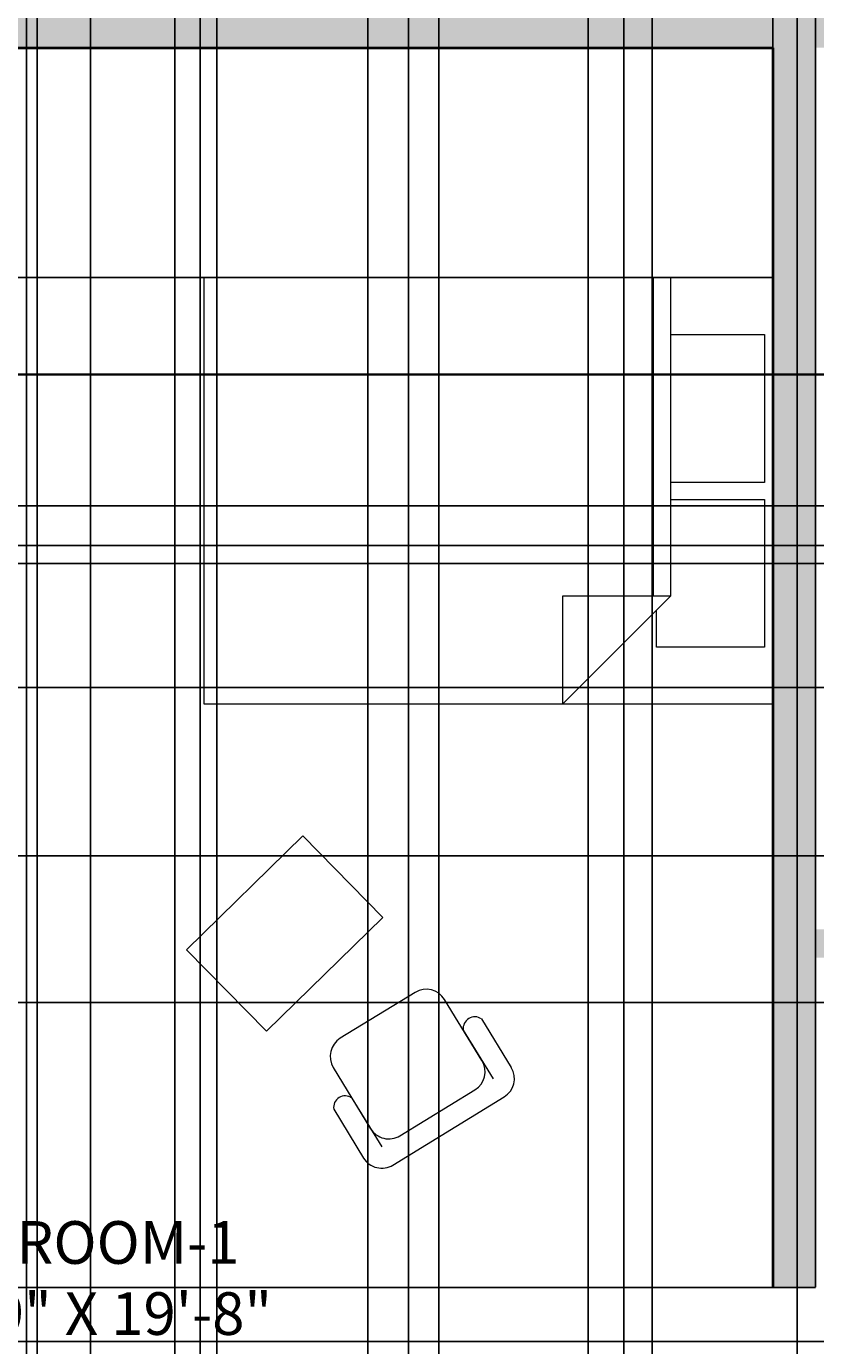
# Model space of a CAD drawing. Units: inches. Extents: x 818 to 1898, y 976 to 2364.
# Tile 43 of 96: x 1512 to 1623, y 1409 to 1594. Entities that reach past the tile are written whole.
import ezdxf

# ---------------------------------------------------------------- set-up
doc = ezdxf.new("R2010")
doc.units = ezdxf.units.IN
doc.header["$LTSCALE"] = 5
doc.header["$MEASUREMENT"] = 0
for name, color, linetype, lineweight in [('A-ANNO-DIMS', 2, 'Continuous', 18), ('A-AREA-IDEN', 7, 'Continuous', 18), ('A-DOOR', 3, 'Continuous', 25), ('A-FURN', 8, 'Continuous', 18), ('A-WALL', 7, 'Continuous', 40)]:
    doc.layers.add(name, color=color, linetype=linetype, lineweight=lineweight)
doc.layers.add('A-WALL-PATT', color=251, linetype='Continuous', lineweight=13, true_color=0x636466)
doc.styles.get("Standard").update_dxf_attribs({"font": 'arial.ttf'})
doc.dimstyles.get("Standard").update_dxf_attribs({"dimtxt": 0.18, "dimasz": 0.18, "dimexe": 0.18, "dimexo": 0.0625, "dimgap": 0.09, "dimtad": 0, "dimtih": 1, "dimtoh": 1, "dimdec": 4, "dimzin": 0, "dimdsep": 46, "dimtxsty": 'Standard', "dimcen": 0.09, "dimadec": 0, "dimazin": 0, "dimtfac": 1, "dimtdec": 4, "dimtofl": 0, "dimtmove": 0, "dimatfit": 3, "dimfxl": 1, "dimtolj": 1, "dimtzin": 0, "dimarcsym": 0})

# ---------------------------------------------------------------- blocks, each defined once
blk = doc.blocks.new('Bed - Queen')
for p, q in [((0, -80.00003), (0, 0)), ((0, 0), (59.99999, 0)), ((59.99999, 0), (59.99999, -80.00003)), ((7.99999, -1.2), (28.79998, -1.2)), ((7.99999, -14.4), (7.99999, -1.2)), ((28.79998, -1.2), (28.79998, -14.4)), ((31.19999, -1.2), (51.99999, -1.2)), ((31.19999, -14.4), (31.19999, -1.2)), ((51.99999, -1.2), (51.99999, -16.4)), ((0, -14.4), (44.8, -14.4)), ((59.99999, -29.6), (44.8, -14.4)), ((44.8, -14.4), (44.8, -29.6)), ((51.99999, -16.4), (46.79936, -16.4)), ((44.8, -16.8), (0, -16.8)), ((44.8, -29.6), (59.99999, -29.6)), ((59.99999, -80.00003), (0, -80.00003))]:
    blk.add_line(p, q)
blk = doc.blocks.new('*D101')
at = {"layer": 'A-ANNO-DIMS', "color": 0, "lineweight": -2, "ltscale": 5, "transparency": 16777216}
for p, q in [((1507.3, 1071.12), (1507.3, 2363.87)), ((1507.48, 2363.69), (1536, 2363.69)), ((1565.3, 2363.69), (1536.78, 2363.69)), ((1565.48, 1071.12), (1565.48, 2363.87))]:
    blk.add_line(p, q, dxfattribs=at)
at = {"layer": 'A-ANNO-DIMS', "color": 0, "ltscale": 5, "transparency": 16777216}
for points in [[(1507.48, 2363.72), (1507.48, 2363.66), (1507.3, 2363.69)], [(1565.3, 2363.72), (1565.3, 2363.66), (1565.48, 2363.69)]]:
    blk.add_solid(points, dxfattribs=at)
at = {"layer": 'Defpoints', "color": 0, "ltscale": 5, "transparency": 16777216}
for p in [(1565.48, 2363.69), (1507.3, 1071.06), (1565.48, 1071.06)]:
    blk.add_point(p, dxfattribs=at)
at = {"layer": 'A-ANNO-DIMS', "color": 0, "ltscale": 5, "transparency": 16777216, "insert": (1536.39, 2363.69), "char_height": 0.18, "attachment_point": 5}
blk.add_mtext('\\A1;58.19', dxfattribs=at)
blk = doc.blocks.new('*D102')
at = {"layer": 'A-ANNO-DIMS', "color": 0, "lineweight": -2, "ltscale": 5, "transparency": 16777216}
for p, q in [((1565.48, 1071.12), (1565.48, 2363.87)), ((1565.66, 2363.69), (1595.63, 2363.69)), ((1626.39, 2363.69), (1596.42, 2363.69)), ((1626.57, 1071.12), (1626.57, 2363.87))]:
    blk.add_line(p, q, dxfattribs=at)
at = {"layer": 'A-ANNO-DIMS', "color": 0, "ltscale": 5, "transparency": 16777216}
for points in [[(1565.66, 2363.72), (1565.66, 2363.66), (1565.48, 2363.69)], [(1626.39, 2363.72), (1626.39, 2363.66), (1626.57, 2363.69)]]:
    blk.add_solid(points, dxfattribs=at)
at = {"layer": 'Defpoints', "color": 0, "ltscale": 5, "transparency": 16777216}
for p in [(1626.57, 2363.69), (1565.48, 1071.06), (1626.57, 1071.06)]:
    blk.add_point(p, dxfattribs=at)
at = {"layer": 'A-ANNO-DIMS', "color": 0, "ltscale": 5, "transparency": 16777216, "insert": (1596.03, 2363.69), "char_height": 0.18, "attachment_point": 5}
blk.add_mtext('\\A1;61.09', dxfattribs=at)
blk = doc.blocks.new('*D116')
at = {"layer": 'A-ANNO-DIMS', "color": 0, "lineweight": -2, "ltscale": 5, "transparency": 16777216}
for p, q in [((1766.29, 1456.81), (818.03, 1456.81)), ((818.21, 1456.63), (818.21, 1417.41)), ((818.21, 1377.84), (818.21, 1417.05)), ((1766.29, 1377.66), (818.03, 1377.66))]:
    blk.add_line(p, q, dxfattribs=at)
at = {"layer": 'A-ANNO-DIMS', "color": 0, "ltscale": 5, "transparency": 16777216}
for points in [[(818.18, 1456.63), (818.24, 1456.63), (818.21, 1456.81)], [(818.18, 1377.84), (818.24, 1377.84), (818.21, 1377.66)]]:
    blk.add_solid(points, dxfattribs=at)
at = {"layer": 'Defpoints', "color": 0, "ltscale": 5, "transparency": 16777216}
for p in [(818.21, 1456.81), (1766.35, 1456.81), (1766.35, 1377.66)]:
    blk.add_point(p, dxfattribs=at)
at = {"layer": 'A-ANNO-DIMS', "color": 0, "ltscale": 5, "transparency": 16777216, "insert": (818.21, 1417.23), "char_height": 0.18, "attachment_point": 5}
blk.add_mtext('\\A1;79.15', dxfattribs=at)
blk = doc.blocks.new('*D117')
at = {"layer": 'A-ANNO-DIMS', "color": 0, "lineweight": -2, "ltscale": 5, "transparency": 16777216}
for p, q in [((1766.29, 1545.18), (818.03, 1545.18)), ((818.21, 1545), (818.21, 1501.18)), ((818.21, 1456.99), (818.21, 1500.81)), ((1766.29, 1456.81), (818.03, 1456.81))]:
    blk.add_line(p, q, dxfattribs=at)
at = {"layer": 'A-ANNO-DIMS', "color": 0, "ltscale": 5, "transparency": 16777216}
for points in [[(818.18, 1545), (818.24, 1545), (818.21, 1545.18)], [(818.18, 1456.99), (818.24, 1456.99), (818.21, 1456.81)]]:
    blk.add_solid(points, dxfattribs=at)
at = {"layer": 'Defpoints', "color": 0, "ltscale": 5, "transparency": 16777216}
for p in [(818.21, 1545.18), (1766.35, 1545.18), (1766.35, 1456.81)]:
    blk.add_point(p, dxfattribs=at)
at = {"layer": 'A-ANNO-DIMS', "color": 0, "ltscale": 5, "transparency": 16777216, "insert": (818.21, 1501), "char_height": 0.18, "attachment_point": 5}
blk.add_mtext('\\A1;88.37', dxfattribs=at)
blk = doc.blocks.new('*D118')
at = {"layer": 'A-ANNO-DIMS', "color": 0, "lineweight": -2, "ltscale": 5, "transparency": 16777216}
for p, q in [((1766.29, 1627.51), (818.03, 1627.51)), ((818.21, 1627.33), (818.21, 1586.53)), ((818.21, 1545.36), (818.21, 1586.16)), ((1766.29, 1545.18), (818.03, 1545.18))]:
    blk.add_line(p, q, dxfattribs=at)
at = {"layer": 'A-ANNO-DIMS', "color": 0, "ltscale": 5, "transparency": 16777216}
for points in [[(818.18, 1627.33), (818.24, 1627.33), (818.21, 1627.51)], [(818.18, 1545.36), (818.24, 1545.36), (818.21, 1545.18)]]:
    blk.add_solid(points, dxfattribs=at)
at = {"layer": 'Defpoints', "color": 0, "ltscale": 5, "transparency": 16777216}
for p in [(818.21, 1627.51), (1766.35, 1627.51), (1766.35, 1545.18)]:
    blk.add_point(p, dxfattribs=at)
at = {"layer": 'A-ANNO-DIMS', "color": 0, "ltscale": 5, "transparency": 16777216, "insert": (818.21, 1586.34), "char_height": 0.18, "attachment_point": 5}
blk.add_mtext('\\A1;82.32', dxfattribs=at)
blk = doc.blocks.new('*D170')
at = {"layer": 'A-ANNO-DIMS', "color": 0, "lineweight": -2, "ltscale": 5, "transparency": 16777216}
for p, q in [((1430.79, 1600.08), (1897.92, 1600.08)), ((1897.74, 1599.9), (1897.74, 1550.76)), ((1897.74, 1501.26), (1897.74, 1550.4)), ((1430.79, 1501.08), (1897.92, 1501.08))]:
    blk.add_line(p, q, dxfattribs=at)
at = {"layer": 'A-ANNO-DIMS', "color": 0, "ltscale": 5, "transparency": 16777216}
for points in [[(1897.71, 1599.9), (1897.77, 1599.9), (1897.74, 1600.08)], [(1897.71, 1501.26), (1897.77, 1501.26), (1897.74, 1501.08)]]:
    blk.add_solid(points, dxfattribs=at)
at = {"layer": 'Defpoints', "color": 0, "ltscale": 5, "transparency": 16777216}
for p in [(1430.73, 1600.08), (1897.74, 1600.08), (1430.73, 1501.08)]:
    blk.add_point(p, dxfattribs=at)
at = {"layer": 'A-ANNO-DIMS', "color": 0, "ltscale": 5, "transparency": 16777216, "insert": (1897.74, 1550.58), "char_height": 0.18, "attachment_point": 5}
blk.add_mtext('\\A1;99', dxfattribs=at)
blk = doc.blocks.new('*D172')
at = {"layer": 'A-ANNO-DIMS', "color": 0, "lineweight": -2, "ltscale": 5, "transparency": 16777216}
for p, q in [((1616.66, 1416.69), (818.03, 1416.69)), ((818.21, 1416.51), (818.21, 1401.87)), ((818.21, 1386.87), (818.21, 1401.5)), ((1616.66, 1386.69), (818.03, 1386.69))]:
    blk.add_line(p, q, dxfattribs=at)
at = {"layer": 'A-ANNO-DIMS', "color": 0, "ltscale": 5, "transparency": 16777216}
for points in [[(818.18, 1416.51), (818.24, 1416.51), (818.21, 1416.69)], [(818.18, 1386.87), (818.24, 1386.87), (818.21, 1386.69)]]:
    blk.add_solid(points, dxfattribs=at)
at = {"layer": 'Defpoints', "color": 0, "ltscale": 5, "transparency": 16777216}
for p in [(818.21, 1416.69), (1616.73, 1416.69), (1616.73, 1386.69)]:
    blk.add_point(p, dxfattribs=at)
at = {"layer": 'A-ANNO-DIMS', "color": 0, "ltscale": 5, "transparency": 16777216, "insert": (818.21, 1401.69), "char_height": 0.18, "attachment_point": 5}
blk.add_mtext('\\A1;30', dxfattribs=at)
blk = doc.blocks.new('*D173')
at = {"layer": 'A-ANNO-DIMS', "color": 0, "lineweight": -2, "ltscale": 5, "transparency": 16777216}
for p, q in [((1622.73, 1463.14), (1622.73, 2363.87)), ((1622.91, 2363.69), (1638.51, 2363.69)), ((1654.55, 2363.69), (1638.94, 2363.69)), ((1654.73, 1463.14), (1654.73, 2363.87))]:
    blk.add_line(p, q, dxfattribs=at)
at = {"layer": 'A-ANNO-DIMS', "color": 0, "ltscale": 5, "transparency": 16777216}
for points in [[(1622.91, 2363.72), (1622.91, 2363.66), (1622.73, 2363.69)], [(1654.55, 2363.72), (1654.55, 2363.66), (1654.73, 2363.69)]]:
    blk.add_solid(points, dxfattribs=at)
at = {"layer": 'Defpoints', "color": 0, "ltscale": 5, "transparency": 16777216}
for p in [(1654.73, 2363.69), (1622.73, 1463.08), (1654.73, 1463.08)]:
    blk.add_point(p, dxfattribs=at)
at = {"layer": 'A-ANNO-DIMS', "color": 0, "ltscale": 5, "transparency": 16777216, "insert": (1638.73, 2363.69), "char_height": 0.18, "attachment_point": 5}
blk.add_mtext('\\A1;32', dxfattribs=at)
blk = doc.blocks.new('*D174')
at = {"layer": 'A-ANNO-DIMS', "color": 0, "lineweight": -2, "ltscale": 5, "transparency": 16777216}
for p, q in [((1616.73, 1416.75), (1616.73, 2363.87)), ((1616.91, 2363.69), (1619.58, 2363.69)), ((1622.55, 2363.69), (1619.87, 2363.69)), ((1622.73, 1416.75), (1622.73, 2363.87))]:
    blk.add_line(p, q, dxfattribs=at)
at = {"layer": 'A-ANNO-DIMS', "color": 0, "ltscale": 5, "transparency": 16777216}
for points in [[(1616.91, 2363.72), (1616.91, 2363.66), (1616.73, 2363.69)], [(1622.55, 2363.72), (1622.55, 2363.66), (1622.73, 2363.69)]]:
    blk.add_solid(points, dxfattribs=at)
at = {"layer": 'Defpoints', "color": 0, "ltscale": 5, "transparency": 16777216}
for p in [(1622.73, 2363.69), (1616.73, 1416.69), (1622.73, 1416.69)]:
    blk.add_point(p, dxfattribs=at)
at = {"layer": 'A-ANNO-DIMS', "color": 0, "ltscale": 5, "transparency": 16777216, "insert": (1619.73, 2363.69), "char_height": 0.18, "attachment_point": 5}
blk.add_mtext('\\A1;6', dxfattribs=at)
blk = doc.blocks.new('*D177')
at = {"layer": 'A-ANNO-DIMS', "color": 0, "lineweight": -2, "ltscale": 5, "transparency": 16777216}
for p, q in [((1559.73, 1647.52), (1559.73, 975.66)), ((1569.73, 1647.52), (1569.73, 975.66)), ((1559.91, 975.84), (1564.52, 975.84)), ((1569.55, 975.84), (1564.94, 975.84))]:
    blk.add_line(p, q, dxfattribs=at)
at = {"layer": 'A-ANNO-DIMS', "color": 0, "ltscale": 5, "transparency": 16777216}
for points in [[(1559.91, 975.87), (1559.91, 975.81), (1559.73, 975.84)], [(1569.55, 975.87), (1569.55, 975.81), (1569.73, 975.84)]]:
    blk.add_solid(points, dxfattribs=at)
at = {"layer": 'Defpoints', "color": 0, "ltscale": 5, "transparency": 16777216}
for p in [(1559.73, 1647.58), (1569.73, 1647.58), (1569.73, 975.84)]:
    blk.add_point(p, dxfattribs=at)
at = {"layer": 'A-ANNO-DIMS', "color": 0, "ltscale": 5, "transparency": 16777216, "insert": (1564.73, 975.84), "char_height": 0.18, "attachment_point": 5}
blk.add_mtext('\\A1;10', dxfattribs=at)
blk = doc.blocks.new('*D180')
at = {"layer": 'A-ANNO-DIMS', "color": 0, "lineweight": -2, "ltscale": 5, "transparency": 16777216}
for p, q in [((1599.73, 1639.52), (1599.73, 975.66)), ((1669.73, 1639.52), (1669.73, 975.66)), ((1599.91, 975.84), (1634.51, 975.84)), ((1669.55, 975.84), (1634.94, 975.84))]:
    blk.add_line(p, q, dxfattribs=at)
at = {"layer": 'A-ANNO-DIMS', "color": 0, "ltscale": 5, "transparency": 16777216}
for points in [[(1599.91, 975.87), (1599.91, 975.81), (1599.73, 975.84)], [(1669.55, 975.87), (1669.55, 975.81), (1669.73, 975.84)]]:
    blk.add_solid(points, dxfattribs=at)
at = {"layer": 'Defpoints', "color": 0, "ltscale": 5, "transparency": 16777216}
for p in [(1599.73, 1639.58), (1669.73, 1639.58), (1669.73, 975.84)]:
    blk.add_point(p, dxfattribs=at)
at = {"layer": 'A-ANNO-DIMS', "color": 0, "ltscale": 5, "transparency": 16777216, "insert": (1634.73, 975.84), "char_height": 0.18, "attachment_point": 5}
blk.add_mtext('\\A1;70', dxfattribs=at)
blk = doc.blocks.new('*D182')
at = {"layer": 'A-ANNO-DIMS', "color": 0, "lineweight": -2, "ltscale": 5, "transparency": 16777216}
for p, q in [((1463.73, 1687.02), (1463.73, 975.66)), ((1559.73, 1687.02), (1559.73, 975.66)), ((1463.91, 975.84), (1511.51, 975.84)), ((1559.55, 975.84), (1511.94, 975.84))]:
    blk.add_line(p, q, dxfattribs=at)
at = {"layer": 'A-ANNO-DIMS', "color": 0, "ltscale": 5, "transparency": 16777216}
for points in [[(1463.91, 975.87), (1463.91, 975.81), (1463.73, 975.84)], [(1559.55, 975.87), (1559.55, 975.81), (1559.73, 975.84)]]:
    blk.add_solid(points, dxfattribs=at)
at = {"layer": 'Defpoints', "color": 0, "ltscale": 5, "transparency": 16777216}
for p in [(1463.73, 1687.08), (1559.73, 1687.08), (1559.73, 975.84)]:
    blk.add_point(p, dxfattribs=at)
at = {"layer": 'A-ANNO-DIMS', "color": 0, "ltscale": 5, "transparency": 16777216, "insert": (1511.73, 975.84), "char_height": 0.18, "attachment_point": 5}
blk.add_mtext('\\A1;96', dxfattribs=at)
blk = doc.blocks.new('*D187')
at = {"layer": 'A-ANNO-DIMS', "color": 0, "lineweight": -2, "ltscale": 5, "transparency": 16777216}
for p, q in [((1705.66, 1545.08), (818.03, 1545.08)), ((818.21, 1544.9), (818.21, 1533.26)), ((818.21, 1521.26), (818.21, 1532.9)), ((1705.66, 1521.08), (818.03, 1521.08))]:
    blk.add_line(p, q, dxfattribs=at)
at = {"layer": 'A-ANNO-DIMS', "color": 0, "ltscale": 5, "transparency": 16777216}
for points in [[(818.18, 1544.9), (818.24, 1544.9), (818.21, 1545.08)], [(818.18, 1521.26), (818.24, 1521.26), (818.21, 1521.08)]]:
    blk.add_solid(points, dxfattribs=at)
at = {"layer": 'Defpoints', "color": 0, "ltscale": 5, "transparency": 16777216}
for p in [(818.21, 1545.08), (1705.73, 1545.08), (1705.73, 1521.08)]:
    blk.add_point(p, dxfattribs=at)
at = {"layer": 'A-ANNO-DIMS', "color": 0, "ltscale": 5, "transparency": 16777216, "insert": (818.21, 1533.08), "char_height": 0.18, "attachment_point": 5}
blk.add_mtext('\\A1;24', dxfattribs=at)
blk = doc.blocks.new('*D194')
at = {"layer": 'A-ANNO-DIMS', "color": 0, "lineweight": -2, "ltscale": 5, "transparency": 16777216}
for p, q in [((1616.66, 1591.08), (818.03, 1591.08)), ((818.21, 1590.9), (818.21, 1575.1)), ((818.21, 1558.93), (818.21, 1574.73)), ((1616.66, 1558.75), (818.03, 1558.75))]:
    blk.add_line(p, q, dxfattribs=at)
at = {"layer": 'A-ANNO-DIMS', "color": 0, "ltscale": 5, "transparency": 16777216}
for points in [[(818.18, 1590.9), (818.24, 1590.9), (818.21, 1591.08)], [(818.18, 1558.93), (818.24, 1558.93), (818.21, 1558.75)]]:
    blk.add_solid(points, dxfattribs=at)
at = {"layer": 'Defpoints', "color": 0, "ltscale": 5, "transparency": 16777216}
for p in [(818.21, 1591.08), (1616.73, 1591.08), (1616.73, 1558.75)]:
    blk.add_point(p, dxfattribs=at)
at = {"layer": 'A-ANNO-DIMS', "color": 0, "ltscale": 5, "transparency": 16777216, "insert": (818.21, 1574.92), "char_height": 0.18, "attachment_point": 5}
blk.add_mtext('\\A1;32.326', dxfattribs=at)
blk = doc.blocks.new('*D197')
at = {"layer": 'A-ANNO-DIMS', "color": 0, "lineweight": -2, "ltscale": 5, "transparency": 16777216}
for p, q in [((1457.79, 1526.67), (1897.92, 1526.67)), ((1897.74, 1526.49), (1897.74, 1468.08)), ((1897.74, 1409.3), (1897.74, 1467.71)), ((1457.79, 1409.12), (1897.92, 1409.12))]:
    blk.add_line(p, q, dxfattribs=at)
at = {"layer": 'A-ANNO-DIMS', "color": 0, "ltscale": 5, "transparency": 16777216}
for points in [[(1897.71, 1526.49), (1897.77, 1526.49), (1897.74, 1526.67)], [(1897.71, 1409.3), (1897.77, 1409.3), (1897.74, 1409.12)]]:
    blk.add_solid(points, dxfattribs=at)
at = {"layer": 'Defpoints', "color": 0, "ltscale": 5, "transparency": 16777216}
for p in [(1457.73, 1526.67), (1897.74, 1526.67), (1457.73, 1409.12)]:
    blk.add_point(p, dxfattribs=at)
at = {"layer": 'A-ANNO-DIMS', "color": 0, "ltscale": 5, "transparency": 16777216, "insert": (1897.74, 1467.89), "char_height": 0.18, "attachment_point": 5}
blk.add_mtext('\\A1;117.55', dxfattribs=at)
blk = doc.blocks.new('*D198')
at = {"layer": 'A-ANNO-DIMS', "color": 0, "lineweight": -2, "ltscale": 5, "transparency": 16777216}
for p, q in [((1741.84, 1545.02), (1741.84, 975.66)), ((1430.73, 1346.02), (1430.73, 975.66)), ((1430.91, 975.84), (1585.91, 975.84)), ((1741.66, 975.84), (1586.66, 975.84))]:
    blk.add_line(p, q, dxfattribs=at)
at = {"layer": 'A-ANNO-DIMS', "color": 0, "ltscale": 5, "transparency": 16777216}
for points in [[(1430.91, 975.87), (1430.91, 975.81), (1430.73, 975.84)], [(1741.66, 975.87), (1741.66, 975.81), (1741.84, 975.84)]]:
    blk.add_solid(points, dxfattribs=at)
at = {"layer": 'Defpoints', "color": 0, "ltscale": 5, "transparency": 16777216}
for p in [(1741.84, 1545.08), (1430.73, 1346.08), (1741.84, 975.84)]:
    blk.add_point(p, dxfattribs=at)
at = {"layer": 'A-ANNO-DIMS', "color": 0, "ltscale": 5, "transparency": 16777216, "insert": (1586.28, 975.84), "char_height": 0.18, "attachment_point": 5}
blk.add_mtext('\\A1;311.1', dxfattribs=at)
blk = doc.blocks.new('*D199')
at = {"layer": 'A-ANNO-DIMS', "color": 0, "lineweight": -2, "ltscale": 5, "transparency": 16777216}
for p, q in [((1559.79, 1687.08), (1897.92, 1687.08)), ((1897.74, 1686.9), (1897.74, 1513.15)), ((1897.74, 1339.05), (1897.74, 1512.79)), ((1660.38, 1338.87), (1897.92, 1338.87))]:
    blk.add_line(p, q, dxfattribs=at)
at = {"layer": 'A-ANNO-DIMS', "color": 0, "ltscale": 5, "transparency": 16777216}
for points in [[(1897.71, 1686.9), (1897.77, 1686.9), (1897.74, 1687.08)], [(1897.71, 1339.05), (1897.77, 1339.05), (1897.74, 1338.87)]]:
    blk.add_solid(points, dxfattribs=at)
at = {"layer": 'Defpoints', "color": 0, "ltscale": 5, "transparency": 16777216}
for p in [(1559.73, 1687.08), (1897.74, 1687.08), (1660.31, 1338.87)]:
    blk.add_point(p, dxfattribs=at)
at = {"layer": 'A-ANNO-DIMS', "color": 0, "ltscale": 5, "transparency": 16777216, "insert": (1897.74, 1512.97), "char_height": 0.18, "attachment_point": 5}
blk.add_mtext('\\A1;348.2', dxfattribs=at)
blk = doc.blocks.new('*D201')
at = {"layer": 'A-ANNO-DIMS', "color": 0, "lineweight": -2, "ltscale": 5, "transparency": 16777216}
for p, q in [((1678.27, 1518.56), (818.03, 1518.56)), ((818.21, 1518.38), (818.21, 1498.18)), ((818.21, 1477.61), (818.21, 1497.81)), ((1678.27, 1477.43), (818.03, 1477.43))]:
    blk.add_line(p, q, dxfattribs=at)
at = {"layer": 'A-ANNO-DIMS', "color": 0, "ltscale": 5, "transparency": 16777216}
for points in [[(818.18, 1518.38), (818.24, 1518.38), (818.21, 1518.56)], [(818.18, 1477.61), (818.24, 1477.61), (818.21, 1477.43)]]:
    blk.add_solid(points, dxfattribs=at)
at = {"layer": 'Defpoints', "color": 0, "ltscale": 5, "transparency": 16777216}
for p in [(818.21, 1518.56), (1678.33, 1518.56), (1678.33, 1477.43)]:
    blk.add_point(p, dxfattribs=at)
at = {"layer": 'A-ANNO-DIMS', "color": 0, "ltscale": 5, "transparency": 16777216, "insert": (818.21, 1497.99), "char_height": 0.18, "attachment_point": 5}
blk.add_mtext('\\A1;41.135', dxfattribs=at)
blk = doc.blocks.new('*D214')
at = {"layer": 'A-ANNO-DIMS', "color": 0, "lineweight": -2, "ltscale": 5, "transparency": 16777216}
for p, q in [((1511.73, 1687.02), (1511.73, 975.66)), ((1714.73, 1687.02), (1714.73, 975.66)), ((1511.91, 975.84), (1612.93, 975.84)), ((1714.55, 975.84), (1613.52, 975.84))]:
    blk.add_line(p, q, dxfattribs=at)
at = {"layer": 'A-ANNO-DIMS', "color": 0, "ltscale": 5, "transparency": 16777216}
for points in [[(1511.91, 975.87), (1511.91, 975.81), (1511.73, 975.84)], [(1714.55, 975.87), (1714.55, 975.81), (1714.73, 975.84)]]:
    blk.add_solid(points, dxfattribs=at)
at = {"layer": 'Defpoints', "color": 0, "ltscale": 5, "transparency": 16777216}
for p in [(1511.73, 1687.08), (1714.73, 1687.08), (1714.73, 975.84)]:
    blk.add_point(p, dxfattribs=at)
at = {"layer": 'A-ANNO-DIMS', "color": 0, "ltscale": 5, "transparency": 16777216, "insert": (1613.23, 975.84), "char_height": 0.18, "attachment_point": 5}
blk.add_mtext('\\A1;203', dxfattribs=at)
blk = doc.blocks.new('*D219')
at = {"layer": 'A-ANNO-DIMS', "color": 0, "lineweight": -2, "ltscale": 5, "transparency": 16777216}
for p, q in [((1595.73, 1696.02), (1595.73, 975.66)), ((1599.73, 1696.02), (1599.73, 975.66)), ((1595.91, 975.84), (1597.57, 975.84)), ((1599.55, 975.84), (1597.88, 975.84))]:
    blk.add_line(p, q, dxfattribs=at)
at = {"layer": 'A-ANNO-DIMS', "color": 0, "ltscale": 5, "transparency": 16777216}
for points in [[(1595.91, 975.87), (1595.91, 975.81), (1595.73, 975.84)], [(1599.55, 975.87), (1599.55, 975.81), (1599.73, 975.84)]]:
    blk.add_solid(points, dxfattribs=at)
at = {"layer": 'Defpoints', "color": 0, "ltscale": 5, "transparency": 16777216}
for p in [(1595.73, 1696.08), (1599.73, 1696.08), (1599.73, 975.84)]:
    blk.add_point(p, dxfattribs=at)
at = {"layer": 'A-ANNO-DIMS', "color": 0, "ltscale": 5, "transparency": 16777216, "insert": (1597.73, 975.84), "char_height": 0.18, "attachment_point": 5}
blk.add_mtext('\\A1;4', dxfattribs=at)
blk = doc.blocks.new('*D224')
at = {"layer": 'A-ANNO-DIMS', "color": 0, "lineweight": -2, "ltscale": 5, "transparency": 16777216}
for p, q in [((1520.73, 1837.52), (1520.73, 975.66)), ((1532.59, 1837.52), (1532.59, 975.66)), ((1520.91, 975.84), (1526.2, 975.84)), ((1532.41, 975.84), (1527.11, 975.84))]:
    blk.add_line(p, q, dxfattribs=at)
at = {"layer": 'A-ANNO-DIMS', "color": 0, "ltscale": 5, "transparency": 16777216}
for points in [[(1520.91, 975.87), (1520.91, 975.81), (1520.73, 975.84)], [(1532.41, 975.87), (1532.41, 975.81), (1532.59, 975.84)]]:
    blk.add_solid(points, dxfattribs=at)
at = {"layer": 'Defpoints', "color": 0, "ltscale": 5, "transparency": 16777216}
for p in [(1520.73, 1837.58), (1532.59, 1837.58), (1532.59, 975.84)]:
    blk.add_point(p, dxfattribs=at)
at = {"layer": 'A-ANNO-DIMS', "color": 0, "ltscale": 5, "transparency": 16777216, "insert": (1526.66, 975.84), "char_height": 0.18, "attachment_point": 5}
blk.add_mtext('\\A1;11.868', dxfattribs=at)
blk = doc.blocks.new('*D226')
at = {"layer": 'A-ANNO-DIMS', "color": 0, "lineweight": -2, "ltscale": 5, "transparency": 16777216}
for p, q in [((1536.17, 1774.47), (1536.17, 975.66)), ((1520.73, 1773.02), (1520.73, 975.66)), ((1520.91, 975.84), (1527.99, 975.84)), ((1535.99, 975.84), (1528.9, 975.84))]:
    blk.add_line(p, q, dxfattribs=at)
at = {"layer": 'A-ANNO-DIMS', "color": 0, "ltscale": 5, "transparency": 16777216}
for points in [[(1520.91, 975.87), (1520.91, 975.81), (1520.73, 975.84)], [(1535.99, 975.87), (1535.99, 975.81), (1536.17, 975.84)]]:
    blk.add_solid(points, dxfattribs=at)
at = {"layer": 'Defpoints', "color": 0, "ltscale": 5, "transparency": 16777216}
for p in [(1536.17, 1774.53), (1520.73, 1773.08), (1536.17, 975.84)]:
    blk.add_point(p, dxfattribs=at)
at = {"layer": 'A-ANNO-DIMS', "color": 0, "ltscale": 5, "transparency": 16777216, "insert": (1528.45, 975.84), "char_height": 0.18, "attachment_point": 5}
blk.add_mtext('\\A1;15.445', dxfattribs=at)
blk = doc.blocks.new('*D229')
at = {"layer": 'A-ANNO-DIMS', "color": 0, "lineweight": -2, "ltscale": 5, "transparency": 16777216}
for p, q in [((1599.73, 2044.02), (1599.73, 975.66)), ((1620.14, 2036.06), (1620.14, 975.66)), ((1599.91, 975.84), (1609.47, 975.84)), ((1619.96, 975.84), (1610.4, 975.84))]:
    blk.add_line(p, q, dxfattribs=at)
at = {"layer": 'A-ANNO-DIMS', "color": 0, "ltscale": 5, "transparency": 16777216}
for points in [[(1599.91, 975.87), (1599.91, 975.81), (1599.73, 975.84)], [(1619.96, 975.87), (1619.96, 975.81), (1620.14, 975.84)]]:
    blk.add_solid(points, dxfattribs=at)
at = {"layer": 'Defpoints', "color": 0, "ltscale": 5, "transparency": 16777216}
for p in [(1599.73, 2044.08), (1620.14, 2036.12), (1620.14, 975.84)]:
    blk.add_point(p, dxfattribs=at)
at = {"layer": 'A-ANNO-DIMS', "color": 0, "ltscale": 5, "transparency": 16777216, "insert": (1609.93, 975.84), "char_height": 0.18, "attachment_point": 5}
blk.add_mtext('\\A1;20.416', dxfattribs=at)
blk = doc.blocks.new('*D242')
at = {"layer": 'A-ANNO-DIMS', "color": 0, "lineweight": -2, "ltscale": 5, "transparency": 16777216}
for p, q in [((1488.26, 1948.6), (1488.26, 975.66)), ((1513.23, 1948.6), (1513.23, 975.66)), ((1488.44, 975.84), (1500.35, 975.84)), ((1513.05, 975.84), (1501.14, 975.84))]:
    blk.add_line(p, q, dxfattribs=at)
at = {"layer": 'A-ANNO-DIMS', "color": 0, "ltscale": 5, "transparency": 16777216}
for points in [[(1488.44, 975.87), (1488.44, 975.81), (1488.26, 975.84)], [(1513.05, 975.87), (1513.05, 975.81), (1513.23, 975.84)]]:
    blk.add_solid(points, dxfattribs=at)
at = {"layer": 'Defpoints', "color": 0, "ltscale": 5, "transparency": 16777216}
for p in [(1488.26, 1948.66), (1513.23, 1948.66), (1513.23, 975.84)]:
    blk.add_point(p, dxfattribs=at)
at = {"layer": 'A-ANNO-DIMS', "color": 0, "ltscale": 5, "transparency": 16777216, "insert": (1500.74, 975.84), "char_height": 0.18, "attachment_point": 5}
blk.add_mtext('\\A1;24.97', dxfattribs=at)
blk = doc.blocks.new('*D243')
at = {"layer": 'A-ANNO-DIMS', "color": 0, "lineweight": -2, "ltscale": 5, "transparency": 16777216}
for p, q in [((1451.77, 2020.02), (1451.77, 975.66)), ((1590.73, 2020.02), (1590.73, 975.66)), ((1451.95, 975.84), (1520.79, 975.84)), ((1590.55, 975.84), (1521.7, 975.84))]:
    blk.add_line(p, q, dxfattribs=at)
at = {"layer": 'A-ANNO-DIMS', "color": 0, "ltscale": 5, "transparency": 16777216}
for points in [[(1451.95, 975.87), (1451.95, 975.81), (1451.77, 975.84)], [(1590.55, 975.87), (1590.55, 975.81), (1590.73, 975.84)]]:
    blk.add_solid(points, dxfattribs=at)
at = {"layer": 'Defpoints', "color": 0, "ltscale": 5, "transparency": 16777216}
for p in [(1451.77, 2020.08), (1590.73, 2020.08), (1590.73, 975.84)]:
    blk.add_point(p, dxfattribs=at)
at = {"layer": 'A-ANNO-DIMS', "color": 0, "ltscale": 5, "transparency": 16777216, "insert": (1521.25, 975.84), "char_height": 0.18, "attachment_point": 5}
blk.add_mtext('\\A1;138.96', dxfattribs=at)
blk = doc.blocks.new('*D253')
at = {"layer": 'A-ANNO-DIMS', "color": 0, "lineweight": -2, "ltscale": 5, "transparency": 16777216}
for p, q in [((1485.12, 2053.02), (1485.12, 975.66)), ((1538.52, 2053.02), (1538.52, 975.66)), ((1485.3, 975.84), (1511.42, 975.84)), ((1538.34, 975.84), (1512.21, 975.84))]:
    blk.add_line(p, q, dxfattribs=at)
at = {"layer": 'A-ANNO-DIMS', "color": 0, "ltscale": 5, "transparency": 16777216}
for points in [[(1485.3, 975.87), (1485.3, 975.81), (1485.12, 975.84)], [(1538.34, 975.87), (1538.34, 975.81), (1538.52, 975.84)]]:
    blk.add_solid(points, dxfattribs=at)
at = {"layer": 'Defpoints', "color": 0, "ltscale": 5, "transparency": 16777216}
for p in [(1485.12, 2053.08), (1538.52, 2053.08), (1538.52, 975.84)]:
    blk.add_point(p, dxfattribs=at)
at = {"layer": 'A-ANNO-DIMS', "color": 0, "ltscale": 5, "transparency": 16777216, "insert": (1511.82, 975.84), "char_height": 0.18, "attachment_point": 5}
blk.add_mtext('\\A1;53.39', dxfattribs=at)

msp = doc.modelspace()

# ---------------------------------------------------------------- hatches: boundary and pattern name
at = {"layer": 'A-WALL-PATT', "ltscale": 5}
h = msp.add_hatch(color=256, dxfattribs=at)
h.dxf.hatch_style = 1
h.paths.add_polyline_path([(1267.7252, 1928.9218), (1258.7252, 1928.9218), (1258.7252, 1913.6401), (1250.3029, 1913.6401), (1250.3029, 1878.3919), (1258.7252, 1878.3919), (1258.7252, 1862.9652), (1267.7252, 1862.9652)])
h.paths.add_polyline_path([(1267.7252, 1814.9652), (1258.7252, 1814.9652), (1258.7252, 1755.3321), (1267.7252, 1755.3321)])
h.paths.add_polyline_path([(1463.7251, 1696.0782), (1267.7252, 1696.0782), (1267.7252, 1707.3321), (1258.7252, 1707.3321), (1258.7252, 1700.0782), (1251.9333, 1700.0782), (1251.9333, 1687.0782), (1463.7251, 1687.0782)])
h.paths.add_polyline_path([(1714.7251, 1717.3178), (1705.7251, 1717.3178), (1705.7251, 1696.0782), (1599.7251, 1696.0782), (1599.7251, 1790.0782), (1705.7251, 1790.0782), (1705.7251, 1785.6125), (1714.7251, 1785.6125), (1714.7251, 1827.2125), (1705.7251, 1827.2125), (1705.7251, 1802.0782), (1599.7251, 1802.0782), (1599.7251, 1867.0782), (1705.7251, 1867.0782), (1705.7251, 1857.2125), (1714.7251, 1857.2125), (1714.7251, 1930.0316), (1741.8409, 1930.0316), (1741.8409, 1935.0316), (1714.7251, 1935.0316), (1714.7251, 1957.0338), (1741.8409, 1957.0338), (1741.8409, 1962.0338), (1714.7251, 1962.0338), (1705.7251, 1962.0338), (1705.7251, 1948.0782), (1599.7251, 1948.0782), (1599.7251, 1981.0782), (1590.7251, 1981.0782), (1590.7251, 1941.0782), (1620.7252, 1941.0782), (1705.7251, 1941.0782), (1705.7251, 1876.0782), (1599.7251, 1876.0782), (1599.7251, 1911.0782), (1590.7251, 1911.0782), (1590.7251, 1876.0782), (1429.2252, 1876.0782), (1429.2252, 1867.0782), (1511.7251, 1867.0782), (1528.593, 1867.0782), (1595.7251, 1867.0782), (1595.7251, 1773.0782), (1520.7251, 1773.0782), (1520.7251, 1837.5823), (1532.593, 1837.5823), (1532.593, 1867.0782), (1528.593, 1867.0782), (1528.593, 1841.5823), (1511.7251, 1841.5823), (1511.7251, 1744.9714), (1520.7251, 1744.9714), (1520.7251, 1761.0782), (1595.7251, 1761.0782), (1595.7251, 1696.0782), (1520.7251, 1696.0782), (1520.7251, 1716.0454), (1511.7251, 1716.0454), (1511.7251, 1696.0782), (1511.7251, 1687.0782), (1714.7251, 1687.0782)])
h.paths.add_polyline_path([(1714.7251, 2053.0782), (1714.7251, 2081.1881), (1709.7252, 2081.1881), (1709.7252, 2053.0782), (1681.6446, 2053.0782), (1681.6446, 2081.1881), (1676.6446, 2081.1881), (1676.6446, 2053.0782), (1538.5155, 2053.0782), (1538.5155, 2044.0782), (1590.7251, 2044.0782), (1590.7251, 2011.0782), (1599.7251, 2011.0782), (1599.7251, 2044.0782), (1705.7251, 2044.0782), (1705.7251, 2014.5114), (1714.7251, 2014.5114)])
h.paths.add_polyline_path([(1485.1216, 2053.0782), (1422.02, 2053.0782), (1422.02, 2081.1881), (1413.02, 2081.1881), (1413.02, 2053.0782), (1399.6356, 2053.0782), (1399.6356, 2081.1881), (1390.6356, 2081.1881), (1390.6356, 2053.0782), (1388.0315, 2053.0782), (1388.0315, 2044.0782), (1416.2743, 2044.0782), (1485.1216, 2044.0782)])
h.paths.add_polyline_path([(1330.305, 2053.0782), (1258.7252, 2053.0782), (1258.7252, 2019.2871), (1267.7252, 2019.2871), (1267.7252, 2044.0782), (1330.305, 2044.0782)])
h.paths.add_polyline_path([(1258.7252, 2053.0782), (1214.6577, 2053.0782), (1214.6577, 2044.0782), (1258.7252, 2044.0782)])
h.paths.add_polyline_path([(1214.6577, 2053.0782), (1180.349, 2053.0782), (1180.349, 2044.0782), (1214.6577, 2044.0782)])
h.paths.add_polyline_path([(1714.7251, 1639.5782), (1741.8409, 1639.5782), (1741.8409, 1643.5782), (1714.7251, 1643.5782), (1714.7251, 1649.9029), (1705.7251, 1649.9029), (1705.7251, 1600.0782), (1477.7252, 1600.0782), (1477.7252, 1591.0782), (1520.7251, 1591.0782), (1616.7251, 1591.0782), (1616.7251, 1416.6857), (1622.7251, 1416.6857), (1622.7251, 1463.0782), (1624.7252, 1463.0782), (1624.7252, 1467.0782), (1622.7251, 1467.0782), (1622.7251, 1591.0782), (1705.7251, 1591.0782), (1705.7251, 1545.0782), (1714.7251, 1545.0782), (1741.8409, 1545.0782), (1741.8409, 1549.0782), (1714.7251, 1549.0782), (1714.7251, 1593.9175), (1737.8409, 1593.9175), (1737.8409, 1597.9175), (1714.7251, 1597.9175)])
h.paths.add_polyline_path([(1674.9024, 2060.7419), (1714.7045, 2060.7419), (1714.7045, 2073.1061), (1674.9024, 2073.1061)], flags=25)
h.paths.add_polyline_path([(1394.5468, 2061.6618), (1422.2344, 2061.6618), (1422.2344, 2074.0261), (1394.5468, 2074.0261)], flags=24)

# ---------------------------------------------------------------- linework, layer by layer
at = {"layer": 'A-DOOR'}
msp.add_line((1622.7251, 1416.6857), (1616.7251, 1416.6857), dxfattribs=at)
at = {"layer": 'A-FURN'}
for p, q in [((1566.4109, 1458.2086), (1555.8766, 1451.7589)), ((1575.7973, 1448.623), (1570.5359, 1457.2165)), ((1575.7251, 1454.4862), (1579.9223, 1447.6309)), ((1573.1666, 1452.9197), (1577.3637, 1446.0645)), ((1554.8845, 1447.6339), (1560.1458, 1439.0405)), ((1564.2708, 1438.0484), (1574.8052, 1444.498)), ((1557.5152, 1443.3372), (1561.7123, 1436.4819)), ((1563.2788, 1433.9234), (1578.9302, 1443.5059)), ((1554.9566, 1441.7707), (1559.1537, 1434.9154))]:
    msp.add_line(p, q, dxfattribs=at)
msp.add_lwpolyline([(1550.5894, 1480.2288), (1534.247, 1464.2199), (1545.4967, 1452.7357), (1561.8392, 1468.7446)], close=True, dxfattribs=at)
for centre, radius, start, end in [((1567.9774, 1455.65), 3, 31.476981, 121.476981), ((1574.7949, 1453.1329), 1.6422, 55.497036, 187.456926), ((1557.443, 1449.2004), 3, 121.476981, 211.476981), ((1573.2387, 1447.0565), 3, 301.476981, 31.476981), ((1577.3637, 1446.0645), 3, 301.476981, 31.476981), ((1556.5525, 1442.0367), 1.618, 53.490576, 189.463386), ((1562.7044, 1440.6069), 3, 211.476981, 301.476981), ((1561.7123, 1436.4819), 3, 211.476981, 301.476981)]:
    msp.add_arc(centre, radius, start, end, dxfattribs=at)
at = {"layer": 'A-WALL'}
for p, q in [((1477.7252, 1591.0782), (1520.7251, 1591.0782)), ((1520.7251, 1591.0782), (1616.7251, 1591.0782)), ((1616.7251, 1591.0782), (1616.7251, 1416.6857))]:
    msp.add_line(p, q, dxfattribs=at)

# ---------------------------------------------------------------- block references
at = {"layer": 'A-FURN', "rotation": 270}
msp.add_blockref('Bed - Queen', (1616.7251, 1558.7521), dxfattribs=at)

# ---------------------------------------------------------------- texts
at = {"layer": 'A-AREA-IDEN', "ltscale": 5, "insert": (1492.6678, 1426.0314), "char_height": 6, "attachment_point": 1}
msp.add_mtext_dynamic_manual_height_columns('BED ROOM-1\\P14\'-9" X 19\'-8"', width=118.992422, gutter_width=1, heights=[0], dxfattribs=at)

# ---------------------------------------------------------------- dimensions: what is measured, and where the dimension line sits
at = {"layer": 'A-ANNO-DIMS', "ltscale": 5}
for base, p1, p2, override, picture, middle in [((1565.4835, 2363.6929), (1507.2982, 1071.0552), (1565.4835, 1071.0552), {"dimdec": 2, "dimlfac": 1, "dimrnd": 0, "dimzin": 0, "dimdsep": 46, "dimlunit": 2}, '*D101', (1536.3908, 2363.6929)), ((1626.5748, 2363.6929), (1565.4835, 1071.0552), (1626.5748, 1071.0552), {"dimdec": 2, "dimlfac": 1, "dimrnd": 0, "dimzin": 0, "dimdsep": 46, "dimlunit": 2}, '*D102', (1596.0291, 2363.6929)), ((1622.7251, 2363.6929), (1616.7251, 1416.6857), (1622.7251, 1416.6857), {"dimdec": 0, "dimlfac": 1, "dimrnd": 0, "dimzin": 0, "dimdsep": 46, "dimlunit": 2}, '*D174', (1619.7251, 2363.6929)), ((1654.7251, 2363.6929), (1622.7251, 1463.0782), (1654.7251, 1463.0782), {"dimdec": 0, "dimlfac": 1, "dimrnd": 0, "dimzin": 0, "dimdsep": 46, "dimlunit": 2}, '*D173', (1638.7251, 2363.6929)), ((1538.5155, 975.8433), (1485.1216, 2053.0782), (1538.5155, 2053.0782), {"dimdec": 2, "dimlfac": 1, "dimrnd": 0, "dimzin": 0, "dimdsep": 46, "dimlunit": 2}, '*D253', (1511.8185, 975.8433)), ((1620.14159, 975.84326), (1599.72515, 2044.07824), (1620.14159, 2036.1182), {"dimdec": 3, "dimlfac": 1, "dimrnd": 0, "dimzin": 0, "dimdsep": 46, "dimlunit": 2}, '*D229', (1609.93337, 975.84326)), ((1590.7251, 975.8433), (1451.7698, 2020.0782), (1590.7251, 2020.0782), {"dimdec": 2, "dimlfac": 1, "dimrnd": 0, "dimzin": 0, "dimdsep": 46, "dimlunit": 2}, '*D243', (1521.2475, 975.8433)), ((1513.2306, 975.8433), (1488.2586, 1948.6602), (1513.2306, 1948.6602), {"dimdec": 2, "dimlfac": 1, "dimrnd": 0, "dimzin": 0, "dimdsep": 46, "dimlunit": 2}, '*D242', (1500.7446, 975.8433)), ((1532.593, 975.8433), (1520.7251, 1837.5823), (1532.593, 1837.5823), {"dimdec": 3, "dimlfac": 1, "dimrnd": 0, "dimzin": 0, "dimdsep": 46, "dimlunit": 2}, '*D224', (1526.6591, 975.8433)), ((1536.1698, 975.8433), (1520.7251, 1773.0782), (1536.1698, 1774.5283), {"dimdec": 3, "dimlfac": 1, "dimrnd": 0, "dimzin": 0, "dimdsep": 46, "dimlunit": 2}, '*D226', (1528.4475, 975.8433)), ((1599.7251, 975.8433), (1595.7251, 1696.0782), (1599.7251, 1696.0782), {"dimdec": 0, "dimlfac": 1, "dimrnd": 0, "dimzin": 0, "dimdsep": 46, "dimlunit": 2}, '*D219', (1597.7251, 975.8433)), ((1559.7251, 975.8433), (1463.7251, 1687.0782), (1559.7251, 1687.0782), {"dimdec": 0, "dimlfac": 1, "dimrnd": 0, "dimzin": 0, "dimdsep": 46, "dimlunit": 2}, '*D182', (1511.7251, 975.8433)), ((1714.7251, 975.8433), (1511.7251, 1687.0782), (1714.7251, 1687.0782), {"dimdec": 0, "dimlfac": 1, "dimrnd": 0, "dimzin": 0, "dimdsep": 46, "dimlunit": 2}, '*D214', (1613.2251, 975.8433)), ((1569.7251, 975.8433), (1559.7251, 1647.5782), (1569.7251, 1647.5782), {"dimdec": 0, "dimlfac": 1, "dimrnd": 0, "dimzin": 0, "dimdsep": 46, "dimlunit": 2}, '*D177', (1564.7251, 975.8433)), ((1669.7251, 975.8433), (1599.7251, 1639.5782), (1669.7251, 1639.5782), {"dimdec": 0, "dimlfac": 1, "dimrnd": 0, "dimzin": 0, "dimdsep": 46, "dimlunit": 2}, '*D180', (1634.7251, 975.8433)), ((1741.8409, 975.8433), (1430.7251, 1346.0782), (1741.8409, 1545.0782), {"dimdec": 1, "dimlfac": 1, "dimrnd": 0, "dimzin": 0, "dimdsep": 46, "dimlunit": 2}, '*D198', (1586.283, 975.8433))]:
    dim = msp.add_linear_dim(base=base, p1=p1, p2=p2, dimstyle='Standard', override=override, dxfattribs=at)
    dim.commit()
    dim.dimension.update_dxf_attribs({"geometry": picture, "text_midpoint": middle})
for base, p1, p2, override, picture, middle in [((1897.736, 1687.0782), (1660.3141, 1338.8654), (1559.7251, 1687.0782), {"dimdec": 1, "dimlfac": 1, "dimrnd": 0, "dimzin": 0, "dimdsep": 46, "dimlunit": 2}, '*D199', (1897.736, 1512.9718)), ((818.2059, 1627.5052), (1766.3524, 1545.1827), (1766.3524, 1627.5052), {"dimdec": 2, "dimlfac": 1, "dimrnd": 0, "dimzin": 0, "dimdsep": 46, "dimlunit": 2}, '*D118', (818.2059, 1586.3439)), ((1897.736, 1600.0782), (1430.7251, 1501.0782), (1430.7251, 1600.0782), {"dimdec": 0, "dimlfac": 1, "dimrnd": 0, "dimzin": 0, "dimdsep": 46, "dimlunit": 2}, '*D170', (1897.736, 1550.5782)), ((818.2059, 1591.0782), (1616.7251, 1558.7521), (1616.7251, 1591.0782), {"dimdec": 3, "dimlfac": 1, "dimrnd": 0, "dimzin": 0, "dimdsep": 46, "dimlunit": 2}, '*D194', (818.2059, 1574.9152)), ((818.2059, 1545.1827), (1766.3524, 1456.8088), (1766.3524, 1545.1827), {"dimdec": 2, "dimlfac": 1, "dimrnd": 0, "dimzin": 0, "dimdsep": 46, "dimlunit": 2}, '*D117', (818.2059, 1500.9957)), ((818.2059, 1545.0782), (1705.7251, 1521.0782), (1705.7251, 1545.0782), {"dimdec": 0, "dimlfac": 1, "dimrnd": 0, "dimzin": 0, "dimdsep": 46, "dimlunit": 2}, '*D187', (818.2059, 1533.0782)), ((1897.736, 1526.6712), (1457.7251, 1409.1177), (1457.7251, 1526.6712), {"dimdec": 2, "dimlfac": 1, "dimrnd": 0, "dimzin": 0, "dimdsep": 46, "dimlunit": 2}, '*D197', (1897.736, 1467.8945)), ((818.2059, 1518.5611), (1678.3302, 1477.4261), (1678.3302, 1518.5611), {"dimdec": 3, "dimlfac": 1, "dimrnd": 0, "dimzin": 0, "dimdsep": 46, "dimlunit": 2}, '*D201', (818.2059, 1497.9936)), ((818.2059, 1456.8088), (1766.3524, 1377.6564), (1766.3524, 1456.8088), {"dimdec": 2, "dimlfac": 1, "dimrnd": 0, "dimzin": 0, "dimdsep": 46, "dimlunit": 2}, '*D116', (818.2059, 1417.2326)), ((818.2059, 1416.6857), (1616.7251, 1386.6857), (1616.7251, 1416.6857), {"dimdec": 0, "dimlfac": 1, "dimrnd": 0, "dimzin": 0, "dimdsep": 46, "dimlunit": 2}, '*D172', (818.2059, 1401.6857))]:
    dim = msp.add_linear_dim(base=base, p1=p1, p2=p2, angle=90, dimstyle='Standard', override=override, dxfattribs=at)
    dim.commit()
    dim.dimension.update_dxf_attribs({"geometry": picture, "text_midpoint": middle})

doc.saveas('drawing.dxf')
